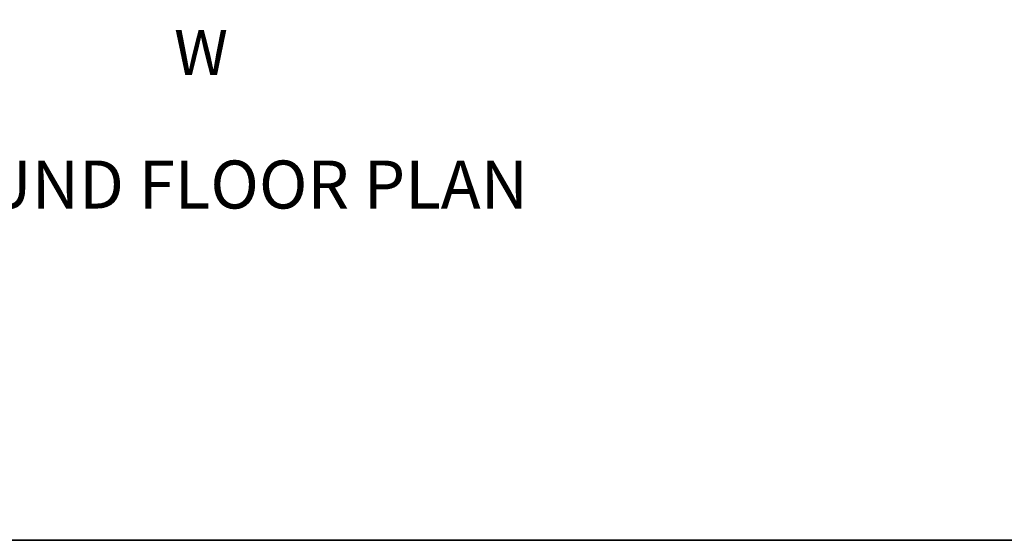
# Model space of a CAD drawing. Units: inches. Extents: x -31485 to -28799, y 18003 to 19130.
# Tile 2 of 15: x -30999 to -30670, y 18003 to 18176. Entities that reach past the tile are written whole.
import ezdxf

# ---------------------------------------------------------------- set-up
doc = ezdxf.new("R2010")
doc.units = ezdxf.units.IN
doc.layers.add('A-ANNO-TEXT', color=7, linetype='Continuous', lineweight=18)
doc.layers.add('A-ANNO-TTLB', color=7, linetype='Continuous', lineweight=35)
doc.styles.get("Standard").update_dxf_attribs({"font": 'arial.ttf'})

msp = doc.modelspace()

# ---------------------------------------------------------------- linework, layer by layer
at = {"layer": 'A-ANNO-TTLB'}
msp.add_lwpolyline([(-31485.09529421644, 19129.94040955191), (-28798.6381181599, 19129.94040955191), (-28798.6381181599, 18002.86338091846), (-31485.09529421644, 18002.86338091846)], close=True, dxfattribs=at)

# ---------------------------------------------------------------- texts
at = {"layer": 'A-ANNO-TEXT', "attachment_point": 1}
for s, width, insert, char_height in [('{W}', 638.5489795821377, (-30947.05712939114, 18173.00259674427), 15), ('{GROUND FLOOR PLAN}', 1323.91503037831, (-31055.39833918592, 18129.45743188856), 16)]:
    msp.add_mtext_dynamic_manual_height_columns(s, width=width, gutter_width=12.5, heights=[0], dxfattribs=dict(at, insert=insert, char_height=char_height))

doc.saveas('drawing.dxf')
